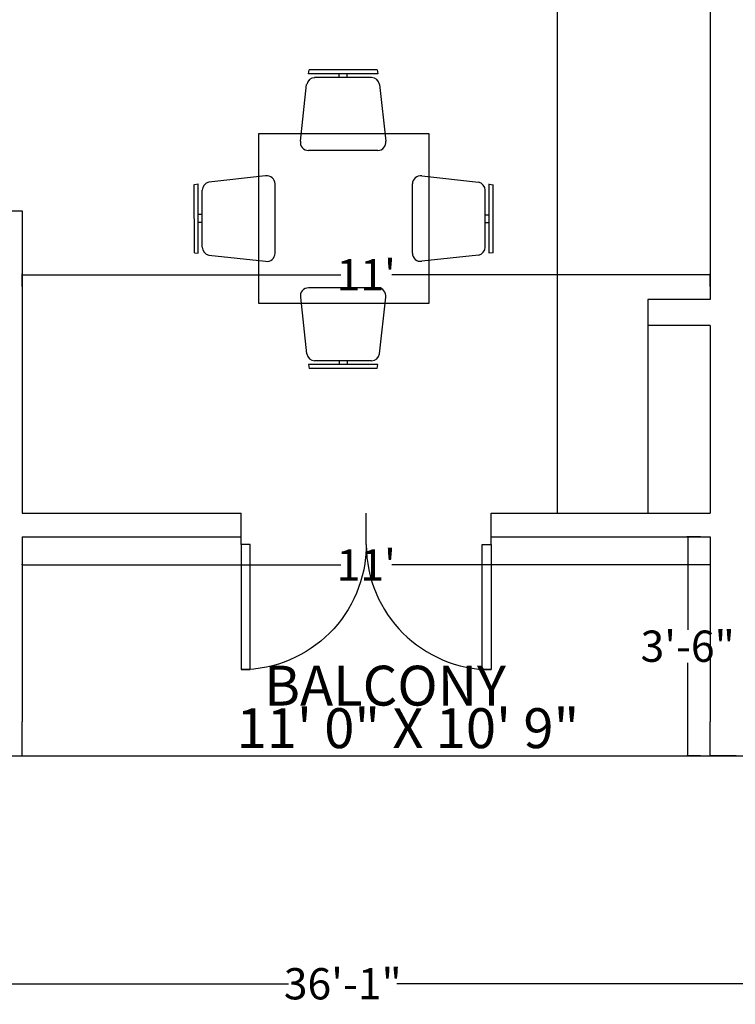
# Model space of a CAD drawing. Units: inches. Extents: x -113 to 5399, y -1393 to 3302.
# Tile 24 of 40: x 3844 to 3982, y -154 to 34. Entities that reach past the tile are written whole.
import ezdxf

# ---------------------------------------------------------------- set-up
doc = ezdxf.new("R2010")
doc.units = ezdxf.units.IN
doc.header["$MEASUREMENT"] = 0
for name, color, linetype, lineweight in [('A-ANNO-DIMS', 254, 'Continuous', 18), ('A-AREA-IDEN', 4, 'Continuous', 18), ('doors', 2, 'Continuous', 25), ('furniture', 131, 'Continuous', 18), ('walls', 1, 'Continuous', 25)]:
    doc.layers.add(name, color=color, linetype=linetype, lineweight=lineweight)
doc.layers.add('B-FURNITURE', color=22, linetype='Continuous')
doc.styles.get("Standard").update_dxf_attribs({"font": 'arial.ttf'})
doc.dimstyles.get("Standard").update_dxf_attribs({"dimtxt": 6, "dimasz": 0.18, "dimexe": 0.18, "dimexo": 0.0625, "dimgap": 0.09, "dimtad": 0, "dimtih": 1, "dimtoh": 1, "dimdec": 1, "dimzin": 0, "dimdsep": 46, "dimlunit": 4, "dimtxsty": 'Standard', "dimblk": 'ARCHTICK', "dimcen": 0.09, "dimadec": 0, "dimazin": 0, "dimtfac": 1, "dimtdec": 1, "dimtofl": 0, "dimtmove": 0, "dimatfit": 3, "dimfxl": 1, "dimtolj": 1, "dimtzin": 0, "dimarcsym": 0})

# ---------------------------------------------------------------- blocks, each defined once
blk = doc.blocks.new('*U2')
for p, q in [((0, 0), (0, -6)), ((24, 0), (24, -6))]:
    blk.add_line(p, q)
blk.add_lwpolyline([(0, 0), (0, 24), (1.75, 24), (1.75, 0)], close=True)
blk.add_arc((0, 0), 24, 0, 90)
blk = doc.blocks.new('A$C6ACA79D1')
at = {"layer": 'B-FURNITURE'}
for p, q in [((-0.5034, 0.0535), (-0.8012, -0.2442)), ((-0.4835, 0.0392), (-0.7869, -0.2642)), ((-0.5034, 0.0535), (-0.4835, 0.0392)), ((-0.4291, 0.0003), (-0.1547, -0.2204)), ((0.7869, -0.259), (0.4835, 0.0444)), ((0.4842, 0.0434), (0.5041, 0.0577)), ((0.7427, -0.249), (0.4935, 0.0002)), ((0.8012, -0.239), (0.5034, 0.0587)), ((-0.4935, -0.005), (-0.7427, -0.2542)), ((-0.601, -0.1125), (-0.6181, -0.0954)), ((0.601, -0.1073), (0.6181, -0.0902)), ((-0.6352, -0.1467), (-0.6523, -0.1296)), ((0.6352, -0.1415), (0.6523, -0.1244)), ((0.8012, -0.239), (0.7869, -0.259)), ((-0.7859, -0.2635), (-0.8002, -0.2436)), ((-0.1485, -0.2964), (-0.4513, -0.5992)), ((0.4513, -0.594), (0.1485, -0.2912)), ((0.748, -0.3133), (0.5273, -0.5877)), ((-0.1485, -1.1937), (-0.4513, -0.8909)), ((0.4513, -0.8961), (0.1485, -1.199)), ((0.748, -1.1768), (0.5273, -0.9024)), ((-0.5034, -1.5436), (-0.8012, -1.2459)), ((-0.7859, -1.2266), (-0.8002, -1.2466)), ((-0.4835, -1.5293), (-0.7869, -1.226)), ((-0.4935, -1.4851), (-0.7427, -1.236)), ((-0.4291, -1.4904), (-0.1547, -1.2698)), ((0.7869, -1.2312), (0.4835, -1.5346)), ((0.7427, -1.2412), (0.4935, -1.4903)), ((0.8012, -1.2511), (0.5034, -1.5488)), ((0.8012, -1.2511), (0.7869, -1.2312)), ((-0.6352, -1.3434), (-0.6523, -1.3605)), ((-0.601, -1.3776), (-0.6181, -1.3948)), ((0.601, -1.3829), (0.6181, -1.4)), ((0.6352, -1.3486), (0.6523, -1.3657)), ((-0.5034, -1.5436), (-0.4835, -1.5293)), ((0.4842, -1.5336), (0.5041, -1.5478))]:
    blk.add_line(p, q, dxfattribs=at)
at = {"layer": 'B-FURNITURE', "ltscale": 300}
for p, q in [((0.1547, -0.2152), (0.4291, 0.0055)), ((-0.5273, -0.593), (-0.748, -0.3186)), ((-0.5273, -0.8972), (-0.748, -1.1716)), ((0.1547, -1.275), (0.4291, -1.4956))]:
    blk.add_line(p, q, dxfattribs=at)
blk.add_lwpolyline([(-0.7425, -0.7425), (0, 0), (0.7425, -0.7425), (0, -1.4849)], close=True, dxfattribs=at)
at = {"layer": 'B-FURNITURE', "ltscale": 400}
for centre, start, end in [((-0.4582, -0.0403), 54.40695, 135), ((0.4589, -0.0361), 45, 125.59305), ((-0.7063, -0.2888), 135, 215.59305), ((0.7073, -0.2843), 324.40695, 45), ((-0.7063, -1.2013), 144.40695, 225), ((0.7073, -1.2059), 315, 35.59305), ((-0.4582, -1.4498), 225, 305.59305), ((0.4589, -1.454), 234.40695, 315)]:
    blk.add_arc(centre, 0.0499, start, end, dxfattribs=at)
at = {"layer": 'B-FURNITURE', "ltscale": 300}
for centre, start, end in [((-0.1838, -0.261), 315, 54.40695), ((0.1838, -0.2558), 125.59305, 225), ((-0.4866, -0.5639), 215.59305, 315), ((0.4866, -0.5586), 225, 324.40695), ((-0.4866, -0.9263), 45, 144.40695), ((0.4866, -0.9315), 35.59305, 135), ((-0.1838, -1.2291), 305.59305, 45), ((0.1838, -1.2343), 135, 234.40695)]:
    blk.add_arc(centre, 0.05, start, end, dxfattribs=at)
blk = doc.blocks.new('_ArchTick')
at = {"color": 0, "linetype": 'ByBlock', "const_width": 0.15}
blk.add_lwpolyline([(-0.5, -0.5), (0.5, 0.5)], dxfattribs=at)
blk = doc.blocks.new('*D99')
at = {"layer": 'A-ANNO-DIMS', "color": 0, "lineweight": -2, "transparency": 16777216}
for p, q in [((3689.73, -100.29), (3689.73, -150.66)), ((4122.73, -100.29), (4122.73, -150.66)), ((3689.73, -150.48), (3895.84, -150.48)), ((4122.73, -150.48), (3916.62, -150.48))]:
    blk.add_line(p, q, dxfattribs=at)
at = {"layer": 'Defpoints', "color": 0, "transparency": 16777216}
for p in [(3689.73, -100.22), (4122.73, -100.22), (4122.73, -150.48)]:
    blk.add_point(p, dxfattribs=at)
at = {"layer": 'A-ANNO-DIMS', "color": 0, "lineweight": -2, "transparency": 16777216, "xscale": 0.18, "yscale": 0.18, "zscale": 0.18, "rotation": 180}
blk.add_blockref('_ArchTick', (3689.73, -150.48), dxfattribs=at)
at = {"layer": 'A-ANNO-DIMS', "color": 0, "lineweight": -2, "transparency": 16777216, "xscale": 0.18, "yscale": 0.18, "zscale": 0.18}
blk.add_blockref('_ArchTick', (4122.73, -150.48), dxfattribs=at)
at = {"layer": 'A-ANNO-DIMS', "color": 0, "transparency": 16777216, "insert": (3906.23, -150.48), "char_height": 6, "attachment_point": 5}
blk.add_mtext('\\A1;36\'-1"', dxfattribs=at)
blk = doc.blocks.new('*D97')
at = {"layer": 'A-ANNO-DIMS', "color": 0, "lineweight": -2, "transparency": 16777216}
for p, q in [((3974.87, -64.72), (3972.22, -64.72)), ((3972.4, -64.72), (3972.4, -82.57)), ((3972.4, -106.72), (3972.4, -88.88)), ((3974.87, -106.72), (3972.22, -106.72))]:
    blk.add_line(p, q, dxfattribs=at)
at = {"layer": 'Defpoints', "color": 0, "transparency": 16777216}
for p in [(3974.93, -64.72), (3972.4, -106.72), (3974.93, -106.72)]:
    blk.add_point(p, dxfattribs=at)
at = {"layer": 'A-ANNO-DIMS', "color": 0, "lineweight": -2, "transparency": 16777216, "xscale": 0.18, "yscale": 0.18, "zscale": 0.18}
for p, rotation in [((3972.4, -64.72), 90), ((3972.4, -106.72), 270)]:
    blk.add_blockref('_ArchTick', p, dxfattribs=dict(at, rotation=rotation))
at = {"layer": 'A-ANNO-DIMS', "color": 0, "transparency": 16777216, "insert": (3972.4, -85.72), "char_height": 6, "attachment_point": 5}
blk.add_mtext('\\A1;3\'-6"', dxfattribs=at)
blk = doc.blocks.new('*D98')
at = {"layer": 'A-ANNO-DIMS', "color": 0, "lineweight": -2, "transparency": 16777216}
for p, q in [((3844.73, -70.08), (3844.73, -69.96)), ((3844.73, -70.14), (3905.83, -70.14)), ((3976.73, -70.14), (3915.63, -70.14)), ((3976.73, -70.08), (3976.73, -69.96))]:
    blk.add_line(p, q, dxfattribs=at)
at = {"layer": 'Defpoints', "color": 0, "transparency": 16777216}
for p in [(3844.73, -70.14), (3976.73, -70.14), (3976.73, -70.14)]:
    blk.add_point(p, dxfattribs=at)
at = {"layer": 'A-ANNO-DIMS', "color": 0, "lineweight": -2, "transparency": 16777216, "xscale": 0.18, "yscale": 0.18, "zscale": 0.18, "rotation": 180}
blk.add_blockref('_ArchTick', (3844.73, -70.14), dxfattribs=at)
at = {"layer": 'A-ANNO-DIMS', "color": 0, "lineweight": -2, "transparency": 16777216, "xscale": 0.18, "yscale": 0.18, "zscale": 0.18}
blk.add_blockref('_ArchTick', (3976.73, -70.14), dxfattribs=at)
at = {"layer": 'A-ANNO-DIMS', "color": 0, "transparency": 16777216, "insert": (3910.73, -70.14), "char_height": 6, "attachment_point": 5}
blk.add_mtext("\\A1;11'", dxfattribs=at)
blk = doc.blocks.new('*D101')
at = {"layer": 'A-ANNO-DIMS', "color": 0, "lineweight": -2, "transparency": 16777216}
for p, q in [((3947.43, 179.78), (3947.43, 62.93)), ((3947.5, 179.78), (3947.61, 179.78)), ((3947.43, -60.22), (3947.43, 56.62)), ((3947.5, -60.22), (3947.61, -60.22))]:
    blk.add_line(p, q, dxfattribs=at)
at = {"layer": 'Defpoints', "color": 0, "transparency": 16777216}
for p in [(3947.43, 179.78), (3947.43, 179.78), (3947.43, -60.22)]:
    blk.add_point(p, dxfattribs=at)
at = {"layer": 'A-ANNO-DIMS', "color": 0, "lineweight": -2, "transparency": 16777216, "xscale": 0.18, "yscale": 0.18, "zscale": 0.18}
for p, rotation in [((3947.43, 179.78), 90), ((3947.43, -60.22), 270)]:
    blk.add_blockref('_ArchTick', p, dxfattribs=dict(at, rotation=rotation))
at = {"layer": 'A-ANNO-DIMS', "color": 0, "transparency": 16777216, "insert": (3947.43, 59.78), "char_height": 6, "attachment_point": 5}
blk.add_mtext("\\A1;20'", dxfattribs=at)
blk = doc.blocks.new('*D102')
at = {"layer": 'A-ANNO-DIMS', "color": 0, "lineweight": -2, "transparency": 16777216}
for p, q in [((3844.73, -16.72), (3844.73, -14.28)), ((3844.73, -14.46), (3905.83, -14.46)), ((3976.73, -14.46), (3915.63, -14.46)), ((3976.73, -16.72), (3976.73, -14.28))]:
    blk.add_line(p, q, dxfattribs=at)
at = {"layer": 'Defpoints', "color": 0, "transparency": 16777216}
for p in [(3844.73, -14.46), (3844.73, -16.78), (3976.73, -16.78)]:
    blk.add_point(p, dxfattribs=at)
at = {"layer": 'A-ANNO-DIMS', "color": 0, "lineweight": -2, "transparency": 16777216, "xscale": 0.18, "yscale": 0.18, "zscale": 0.18, "rotation": 180}
blk.add_blockref('_ArchTick', (3844.73, -14.46), dxfattribs=at)
at = {"layer": 'A-ANNO-DIMS', "color": 0, "lineweight": -2, "transparency": 16777216, "xscale": 0.18, "yscale": 0.18, "zscale": 0.18}
blk.add_blockref('_ArchTick', (3976.73, -14.46), dxfattribs=at)
at = {"layer": 'A-ANNO-DIMS', "color": 0, "transparency": 16777216, "insert": (3910.73, -14.46), "char_height": 6, "attachment_point": 5}
blk.add_mtext("\\A1;11'", dxfattribs=at)
blk = doc.blocks.new('*D210')
at = {"layer": 'A-ANNO-DIMS', "color": 0, "lineweight": -2, "transparency": 16777216}
for p, q in [((3839.79, 561.28), (4159.21, 561.28)), ((4159.03, 561.28), (4159.03, 230.43)), ((4159.03, -106.72), (4159.03, 224.12)), ((3839.79, -106.72), (4159.21, -106.72))]:
    blk.add_line(p, q, dxfattribs=at)
at = {"layer": 'Defpoints', "color": 0, "transparency": 16777216}
for p in [(3839.73, 561.28), (4159.03, 561.28), (3839.73, -106.72)]:
    blk.add_point(p, dxfattribs=at)
at = {"layer": 'A-ANNO-DIMS', "color": 0, "lineweight": -2, "transparency": 16777216, "xscale": 0.18, "yscale": 0.18, "zscale": 0.18}
for p, rotation in [((4159.03, 561.28), 90), ((4159.03, -106.72), 270)]:
    blk.add_blockref('_ArchTick', p, dxfattribs=dict(at, rotation=rotation))
at = {"layer": 'A-ANNO-DIMS', "color": 0, "transparency": 16777216, "insert": (4159.03, 227.28), "char_height": 6, "attachment_point": 5}
blk.add_mtext('\\A1;55\'-8"', dxfattribs=at)

msp = doc.modelspace()

# ---------------------------------------------------------------- linework, layer by layer
at = {"layer": 'walls'}
for p, q in [((3976.73, 55.28), (3976.73, -19.22)), ((3839.73, -2.22), (3844.73, -2.22)), ((3844.73, -2.22), (3844.73, -60.22)), ((3976.73, -19.22), (3964.73, -19.22)), ((3964.73, -19.22), (3964.73, -24.22)), ((3976.73, -24.22), (3964.73, -24.22)), ((3964.73, -24.22), (3964.73, -60.22)), ((3976.73, -24.22), (3976.73, -60.22)), ((3844.73, -60.22), (3886.73, -60.22)), ((3886.73, -64.72), (3886.73, -60.22)), ((3934.73, -60.22), (3976.73, -60.22)), ((3934.73, -64.72), (3934.73, -60.22)), ((3844.73, -64.72), (3844.73, -100.22)), ((3844.73, -64.72), (3886.73, -64.72)), ((3934.73, -64.72), (3976.73, -64.72)), ((3976.73, -64.72), (3976.73, -100.22)), ((3844.73, -106.72), (3844.73, -100.22)), ((3976.73, -106.72), (3976.73, -100.22)), ((3839.73, -106.72), (3844.73, -106.72)), ((3844.73, -106.72), (3976.73, -106.72)), ((3981.73, -106.72), (3976.73, -106.72))]:
    msp.add_line(p, q, dxfattribs=at)

# ---------------------------------------------------------------- block references
at = {"layer": 'doors', "xscale": -1, "rotation": 180}
msp.add_blockref('*U2', (3886.73, -66.22), dxfattribs=at)
at = {"layer": 'doors', "rotation": 180}
msp.add_blockref('*U2', (3934.73, -66.22), dxfattribs=at)
at = {"layer": 'furniture', "xscale": 31.0665876167328, "yscale": 31.0665876167328, "zscale": 31.0665876167328, "rotation": 314.9999999999397}
msp.add_blockref('A$C6ACA79D1', (3922.72, 12.63), dxfattribs=at)

# ---------------------------------------------------------------- texts
at = {"layer": 'A-AREA-IDEN'}
for s, height, p in [('BALCONY', 7.647, (3891.18, -97.11)), ('11\' 0" X 10\' 9"', 7.6473, (3885.85, -105.27))]:
    msp.add_text(s, height=height, dxfattribs=at).set_placement(p)

# ---------------------------------------------------------------- dimensions: what is measured, and where the dimension line sits
at = {"layer": 'A-ANNO-DIMS'}
for base, p1, p2, override, picture, middle in [((4159.03, 561.28), (3839.73, -106.72), (3839.73, 561.28), {"dimdec": 1, "dimlfac": 1, "dimrnd": 0, "dimzin": 1, "dimdsep": 46, "dimlunit": 4, "dimfrac": 2}, '*D210', (4159.03, 227.28)), ((3947.43, 179.78), (3947.43, -60.22), (3947.43, 179.78), {"dimclrd": 0, "dimclre": 0, "dimclrt": 0}, '*D101', (3947.43, 59.78)), ((3972.4, -106.72), (3974.93, -64.72), (3974.93, -106.72), {"dimclrd": 0, "dimclre": 0, "dimclrt": 0}, '*D97', (3972.4, -85.72))]:
    dim = msp.add_linear_dim(base=base, p1=p1, p2=p2, angle=90, dimstyle='Standard', override=override, dxfattribs=at)
    dim.commit()
    dim.dimension.update_dxf_attribs({"geometry": picture, "text_midpoint": middle})
for base, p1, p2, picture, middle in [((3844.73, -14.46), (3976.73, -16.78), (3844.73, -16.78), '*D102', (3910.73, -14.46)), ((3976.73, -70.14), (3844.73, -70.14), (3976.73, -70.14), '*D98', (3910.73, -70.14)), ((4122.73, -150.48), (3689.73, -100.22), (4122.73, -100.22), '*D99', (3906.23, -150.48))]:
    dim = msp.add_linear_dim(base=base, p1=p1, p2=p2, dimstyle='Standard', override={"dimclrd": 0, "dimclre": 0, "dimclrt": 0}, dxfattribs=at)
    dim.commit()
    dim.dimension.update_dxf_attribs({"geometry": picture, "text_midpoint": middle})

doc.saveas('drawing.dxf')
